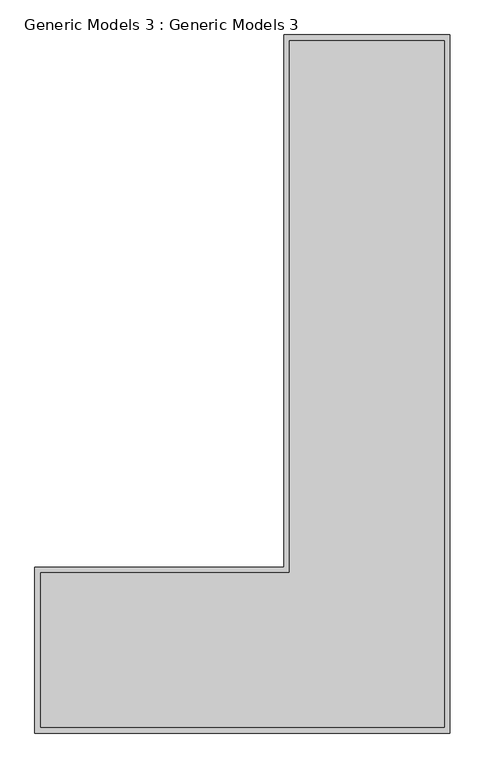
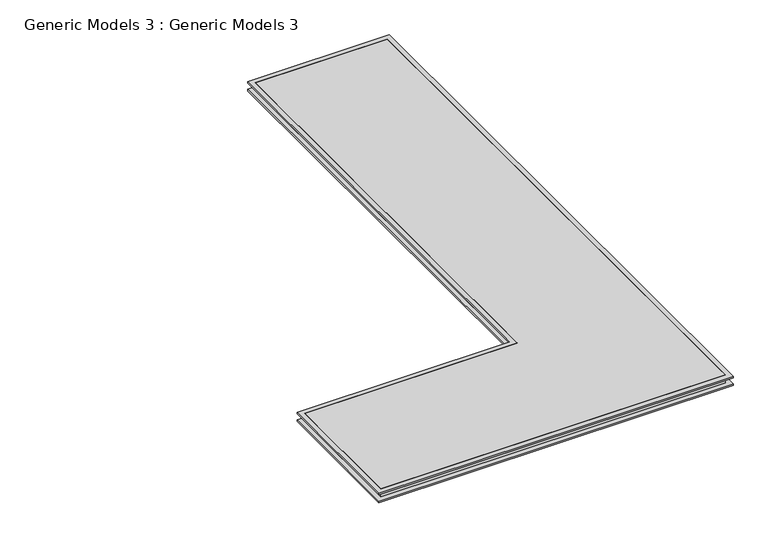
"""IFC4 building model written with IfcOpenShell, lengths in millimetres: proxy geometry, Generic Models 3 : Generic Models 3."""

from ifc_helpers import new_model, si_unit, frame, origin, place, context, project, spatial, polyline, outline, extrude, source, transform, mapped, element, save


def generic_models_3_generic_models_3_71c6270e(model_context):
    return source(origin(), model_context, "Body", "SweptSolid", [
        extrude(outline(polyline([(8543.6590234, -8951.658484), (3014.1557451, -8951.658484), (3014.1557451, -6741.858484), (6333.8590234, -6741.858484), (6333.8590234, 343.6142537), (8543.6590234, 343.6142537), (8543.6590234, -8951.658484)]), holes=[polyline([(6410.0590234, -6818.058484), (3090.3557451, -6818.058484), (3090.3557451, -8875.458484), (8467.4590234, -8875.458484), (8467.4590234, 267.4142537), (6410.0590234, 267.4142537), (6410.0590234, -6818.058484)])]), frame((0.0, 0.0, 7899.4), z_axis=(0.0, 0.0, 1.0), x_axis=(1.0, 0.0, 0.0)), (0.0, 0.0, 1.0), 25.4),
        extrude(outline(polyline([(8543.6590234, -8951.658484), (3014.1557451, -8951.658484), (3014.1557451, -6741.858484), (6333.8590234, -6741.858484), (6333.8590234, 343.6142537), (8543.6590234, 343.6142537), (8543.6590234, -8951.658484)]), holes=[polyline([(6410.0590234, -6818.058484), (3090.3557451, -6818.058484), (3090.3557451, -8875.458484), (8467.4590234, -8875.458484), (8467.4590234, 267.4142537), (6410.0590234, 267.4142537), (6410.0590234, -6818.058484)])]), frame((0.0, 0.0, 7772.4), z_axis=(0.0, 0.0, 1.0), x_axis=(1.0, 0.0, 0.0)), (0.0, 0.0, 1.0), 25.4),
        extrude(outline(polyline([(8467.4590234, -8875.458484), (3090.3557451, -8875.458484), (3090.3557451, -6818.058484), (6410.0590234, -6818.058484), (6410.0590234, 267.4142537), (7324.4590234, 267.4142537), (8467.4590234, 267.4142537), (8467.4590234, -8875.458484)])), frame((0.0, 0.0, 7772.4), z_axis=(0.0, 0.0, 1.0), x_axis=(1.0, 0.0, 0.0)), (0.0, 0.0, 1.0), 152.4),
    ])


if __name__ == "__main__":
    model = new_model("IFC4")
    model_context = context("Model", 3, world=origin())
    ifc_project = project(units=[si_unit("LENGTHUNIT", "METRE", prefix="MILLI")], contexts=[model_context])
    site = spatial("IfcSite", under=ifc_project)
    building = spatial("IfcBuilding", under=site)
    placement = place(None, origin())
    generic_models_3_generic_models_3_shape = generic_models_3_generic_models_3_71c6270e(model_context)
    element("IfcBuildingElementProxy", 1, Name="Generic Models 3 : Generic Models 3", ObjectType="Generic Models 3 : Generic Models 3", at=placement, inside=building, context=model_context, shape_type="MappedRepresentation", body=[
        mapped(generic_models_3_generic_models_3_shape, transform((0.0, 0.0, 0.0), x_axis=(1.0, 0.0, 0.0), y_axis=(0.0, 1.0, 0.0), z_axis=(0.0, 0.0, 1.0))),
    ])
    save(model, "model.ifc")

# Revit data of these elements
# Element 1 (IfcBuildingElementProxy, "Generic Models 3 : Generic Models 3")
#   Materials on its faces: "blk", "Topo cama"
# Materials
#   "blk": class "Generic", colour RGB 0 0 0, transparency 0, Cost = 0
#   "Topo cama": class "Wood", colour RGB 65 50 39, transparency 0
